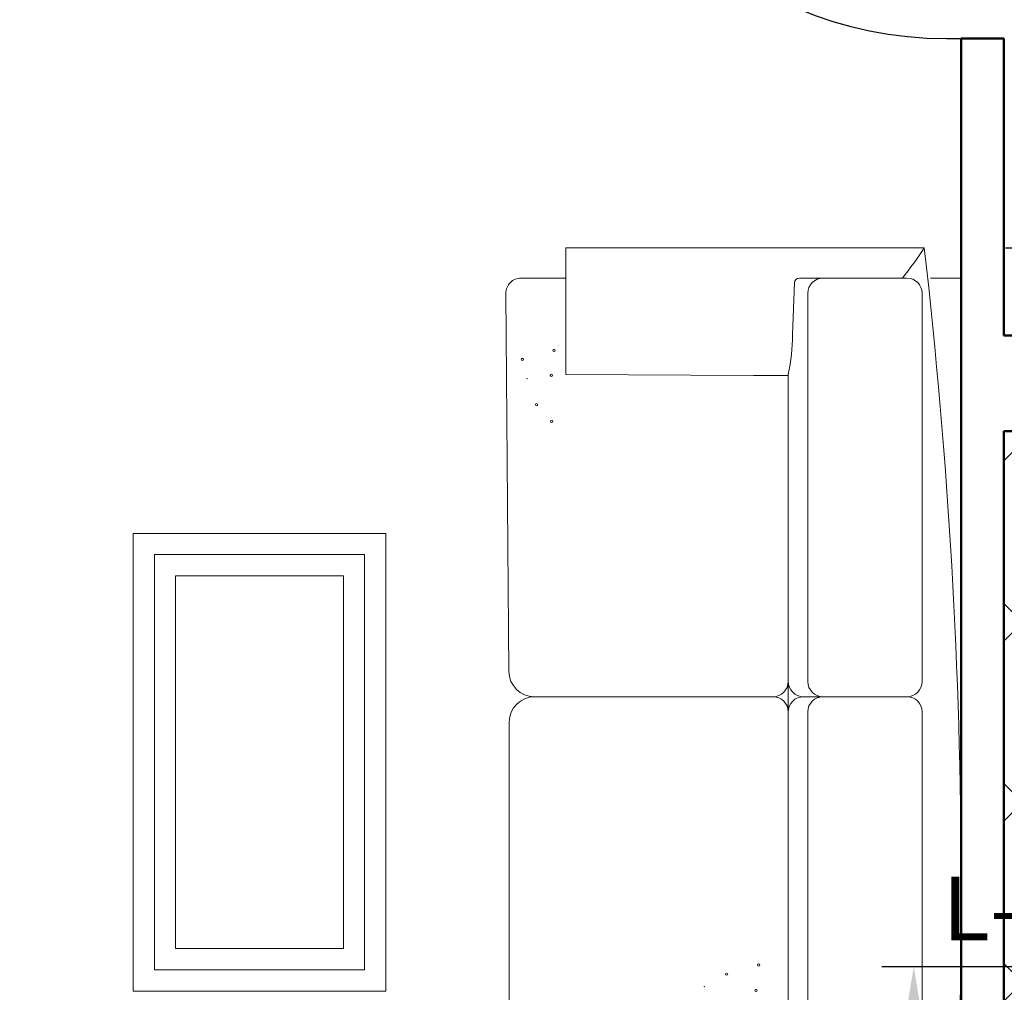
# Model space of a CAD drawing. Units: inches. Extents: x -466983 to 1020, y 324 to 318697.
# Tile 22 of 97: x 721 to 814, y 566 to 658. Entities that reach past the tile are written whole.
import ezdxf

# ---------------------------------------------------------------- set-up
doc = ezdxf.new("R2010")
doc.units = ezdxf.units.IN
doc.header["$MEASUREMENT"] = 0
for name, color, linetype, lineweight in [('A-ANNO-DIMS', 2, 'Continuous', 18), ('A-DOOR', 3, 'Continuous', 25), ('A-FLOR-PATT', 252, 'Continuous', 13), ('A-FURN', 8, 'Continuous', 18), ('A-WALL', 7, 'Continuous', 50)]:
    doc.layers.add(name, color=color, linetype=linetype, lineweight=lineweight)
doc.styles.get("Standard").update_dxf_attribs({"font": 'arial.ttf'})
doc.dimstyles.get("Standard").update_dxf_attribs({"dimtxt": 6, "dimasz": 4, "dimexe": 3, "dimexo": 3, "dimgap": 0.09, "dimtad": 0, "dimtih": 1, "dimtoh": 1, "dimdec": 1, "dimzin": 0, "dimdsep": 46, "dimlunit": 3, "dimtxsty": 'Standard', "dimcen": 0.09, "dimadec": 0, "dimazin": 0, "dimtfac": 1, "dimtdec": 1, "dimtofl": 0, "dimtmove": 0, "dimatfit": 3, "dimfxl": 1, "dimtolj": 1, "dimtzin": 0, "dimarcsym": 0})

# ---------------------------------------------------------------- blocks, each defined once
blk = doc.blocks.new('L Shaped Sofa')
at = {"ltscale": 2}
for p, q in [((2438.01, 846.521), (2438.01, 834.581)), ((2471.772, 846.521), (2438.01, 846.521)), ((2438.01, 843.655), (2433.801, 843.655)), ((2459.543, 843.195), (2459.371, 838.325)), ((2460.02, 843.655), (2462.233, 843.655)), ((2470.142, 843.655), (2462.233, 843.655)), ((2475.263, 843.655), (2472.363, 843.655)), ((2475.263, 843.655), (2475.263, 821.686)), ((2432.653, 806.575), (2432.368, 842.211)), ((2460.8, 842.223), (2460.8, 821.686)), ((2471.575, 842.223), (2471.575, 821.686)), ((2455.692, 834.489), (2438.01, 834.581)), ((2455.692, 834.489), (2458.96, 834.489)), ((2458.96, 834.581), (2458.96, 805.639)), ((2460.8, 805.639), (2460.8, 821.686)), ((2471.575, 805.639), (2471.575, 821.686)), ((2475.263, 723.229), (2475.263, 821.686)), ((2458.96, 802.773), (2458.96, 805.639)), ((2435.071, 804.206), (2435.04, 804.206)), ((2457.527, 804.206), (2435.071, 804.206)), ((2457.527, 804.206), (2457.527, 804.206)), ((2462.233, 804.206), (2460.393, 804.206)), ((2470.142, 804.206), (2462.233, 804.206)), ((2458.96, 739.532), (2458.96, 802.773)), ((2460.8, 737.692), (2460.8, 802.773)), ((2471.575, 769.955), (2471.575, 802.773)), ((2432.683, 769.955), (2432.683, 801.818))]:
    blk.add_line(p, q, dxfattribs=at)
for centre, radius, start, end in [((2441.545, 866.112), 36.021, 321.43275, 327.0519), ((1939.075, 785.436), 536.188, 353.68225, 6.54157), ((2433.801, 842.223), 1.433, 90, 180.45787), ((2460.02, 843.178), 0.478, 90, 177.98163), ((2462.233, 842.223), 1.433, 90, 180), ((2470.142, 842.223), 1.433, 0, 90), ((2441.716, 838.368), 17.655, 347.61307, 359.85818), ((2436.906, 836.857), 0.106, 1.3946, 181.3946), ((2436.906, 836.857), 0.106, 181.3946, 1.3946), ((2433.902, 836.001), 0.106, 1.3946, 181.3946), ((2433.902, 836.001), 0.106, 181.3946, 1.3946), ((2434.341, 834.182), 0.0177, 1.3946, 181.3946), ((2434.341, 834.182), 0.0177, 181.3946, 1.3946), ((2436.655, 834.485), 0.106, 1.3946, 181.3946), ((2436.655, 834.485), 0.106, 181.3946, 1.3946), ((2435.251, 831.737), 0.106, 1.3946, 181.3946), ((2435.251, 831.737), 0.106, 181.3946, 1.3946), ((2436.686, 830.165), 0.106, 1.3946, 181.3946), ((2436.686, 830.165), 0.106, 181.3946, 1.3946), ((2435.04, 806.594), 2.388, 180.45787, 270), ((2457.527, 805.639), 1.433, 270, 0), ((2460.393, 805.639), 1.433, 180, 270), ((2462.233, 805.639), 1.433, 180, 270), ((2470.142, 805.639), 1.433, 270, 0), ((2435.071, 801.818), 2.388, 90, 180), ((2457.527, 802.773), 1.433, 0, 90), ((2460.393, 802.773), 1.433, 90, 180), ((2462.233, 802.773), 1.433, 90, 180), ((2470.142, 802.773), 1.433, 0, 90), ((2453.169, 778.058), 0.106, 1.3946, 181.3946), ((2456.173, 778.913), 0.106, 1.3946, 181.3946), ((2456.173, 778.913), 0.106, 181.3946, 1.3946), ((2453.169, 778.058), 0.106, 181.3946, 1.3946), ((2451.048, 776.875), 0.0177, 1.3946, 181.3946), ((2451.048, 776.875), 0.0177, 181.3946, 1.3946), ((2455.922, 776.541), 0.106, 1.3946, 181.3946), ((2455.922, 776.541), 0.106, 181.3946, 1.3946)]:
    blk.add_arc(centre, radius, start, end, dxfattribs=at)
blk = doc.blocks.new('*U39')
for p, q in [((0, 0), (0, -6)), ((-40, 0), (-40, -6))]:
    blk.add_line(p, q)
blk.add_lwpolyline([(0, 0), (0, 40), (-1.75, 40), (-1.75, 0)], close=True)
blk.add_arc((0, 0), 40, 90, 180)
blk = doc.blocks.new('*D69')
at = {"layer": 'A-ANNO-DIMS', "color": 0, "lineweight": -2, "transparency": 16777216}
for p, q in [((813.968, 636.229), (832.65, 636.229)), ((829.65, 632.229), (829.65, 577.152)), ((829.65, 515.686), (829.65, 570.763)), ((813.968, 511.686), (832.65, 511.686))]:
    blk.add_line(p, q, dxfattribs=at)
at = {"layer": 'A-ANNO-DIMS', "color": 0, "transparency": 16777216}
for points in [[(828.983, 632.229), (830.316, 632.229), (829.65, 636.229)], [(828.983, 515.686), (830.316, 515.686), (829.65, 511.686)]]:
    blk.add_solid(points, dxfattribs=at)
at = {"layer": 'Defpoints', "color": 0, "transparency": 16777216}
for p in [(810.968, 636.229), (829.65, 636.229), (810.968, 511.686)]:
    blk.add_point(p, dxfattribs=at)
at = {"layer": 'A-ANNO-DIMS', "color": 0, "transparency": 16777216, "insert": (829.65, 573.958), "char_height": 6, "attachment_point": 5}
blk.add_mtext('\\A1;L-SOFA 125', dxfattribs=at)
blk = doc.blocks.new('*D97')
at = {"layer": 'A-ANNO-DIMS', "color": 0, "lineweight": -2, "transparency": 16777216}
for p, q in [((823.929, 568.441), (802.329, 568.441)), ((805.329, 564.441), (805.329, 499.545)), ((805.329, 428.441), (805.329, 493.337)), ((823.929, 424.441), (802.329, 424.441))]:
    blk.add_line(p, q, dxfattribs=at)
at = {"layer": 'A-ANNO-DIMS', "color": 0, "transparency": 16777216}
for points in [[(804.662, 564.441), (805.996, 564.441), (805.329, 568.441)], [(804.662, 428.441), (805.996, 428.441), (805.329, 424.441)]]:
    blk.add_solid(points, dxfattribs=at)
at = {"layer": 'Defpoints', "color": 0, "transparency": 16777216}
for p in [(826.929, 568.441), (805.329, 424.441), (826.929, 424.441)]:
    blk.add_point(p, dxfattribs=at)
at = {"layer": 'A-ANNO-DIMS', "color": 0, "transparency": 16777216, "insert": (805.329, 496.441), "char_height": 6, "attachment_point": 5}
blk.add_mtext('\\A1;BIKE 144', dxfattribs=at)

msp = doc.modelspace()

# ---------------------------------------------------------------- hatches: boundary and pattern name
at = {"layer": 'A-FLOR-PATT', "transparency": 33554572}
h = msp.add_hatch(dxfattribs=at)
h.set_pattern_fill('ANSI37', color=256, scale=30)
h.set_pattern_definition([(45, (-1212.4137, -290.035), (-2.6516504, 2.6516504), []), (135, (-1212.4137, -290.035), (-2.6516504, -2.6516504), [])])
h.paths.add_polyline_path([(901.806, 1075.938), (900.614, 1075.938), (900.614, 1065.386), (899.391, 1065.386), (898.091, 1065.386), (892.836, 1058.71, -0.258377), (892.188, 1058.351), (879.985, 1058.351, -0.20177), (879.438, 1058.581), (874.081, 1065.386), (872.781, 1065.386), (871.558, 1065.386), (871.558, 1075.938), (813.806, 1075.938), (813.806, 1044.792), (832.395, 1044.792, -0.394795), (848.66, 1028.536), (848.66, 1009.938), (901.806, 1009.938), (901.806, 1015.938), (901.306, 1015.938), (871.306, 1015.938), (871.306, 1017.25), (871.334, 1017.25, -0.401453), (901.306, 1045.938), (901.806, 1045.938)])
edge = h.paths.add_edge_path(flags=16)
edge.add_line((847.773, 1068.949), (847.773, 1073.709))
edge.add_arc((849.227, 1073.709), 1.454, 90, 180, ccw=False)
edge.add_line((849.227, 1075.163), (864.492, 1075.163))
edge.add_arc((864.492, 1073.709), 1.454, 0, 90, ccw=False)
edge.add_line((865.946, 1073.709), (865.946, 1069.004))
edge.add_arc((832.645, 1068.976), 33.301, -20.61234, 0.04725, ccw=False)
edge.add_ellipse((856.859, 1058.48), major_axis=(0, 10.213), ratio=0.685919, start_angle=100.00884, end_angle=259.99116, ccw=False)
edge.add_arc((881.074, 1068.976), 33.301, 180.04725, 200.61234, ccw=False)
h.paths.add_polyline_path([(853.146, 1066.482), (853.146, 1066.453), (853.146, 1066.453, 0.433107), (852.917, 1066.685), (852.917, 1066.453), (853.146, 1066.453), (853.146, 1066.482), (853.088, 1066.612, 0.697939), (852.7, 1066.453), (852.7, 1066.453), (852.7, 1066.482), (852.917, 1067.001), (852.917, 1066.685, -0.396254)], flags=0)
h.paths.add_polyline_path([(861.019, 1066.482), (861.019, 1066.453), (861.019, 1066.453, 0.416404), (860.802, 1066.685), (860.802, 1066.453), (861.019, 1066.453), (861.019, 1066.482), (860.967, 1066.605, 0.713344), (860.573, 1066.453), (860.573, 1066.453), (860.573, 1066.482), (860.802, 1067.001), (860.802, 1066.685, -0.379973)], flags=0)
edge = h.paths.add_edge_path(flags=0)
edge.add_spline(control_points=[(861.13, 1065.785), (861.466, 1065.248), (861.613, 1065.016), (861.983, 1064.374), (862.192, 1063.944), (862.561, 1063.039), (862.721, 1062.563), (862.987, 1061.578), (863.092, 1061.069), (863.245, 1060.031), (863.293, 1059.503), (863.329, 1058.441), (863.318, 1057.908), (863.237, 1056.852), (863.166, 1056.329), (862.97, 1055.308), (862.843, 1054.81), (862.537, 1053.852), (862.357, 1053.393), (861.951, 1052.525), (861.725, 1052.117), (861.233, 1051.362), (860.967, 1051.016), (860.405, 1050.395), (860.108, 1050.12), (859.494, 1049.646), (859.176, 1049.448), (858.528, 1049.13), (858.197, 1049.011), (857.531, 1048.852), (857.196, 1048.812), (856.525, 1048.812), (856.189, 1048.852), (855.524, 1049.01), (855.193, 1049.129), (854.545, 1049.447), (854.227, 1049.645), (853.612, 1050.118), (853.316, 1050.393), (852.753, 1051.014), (852.487, 1051.36), (851.995, 1052.114), (851.769, 1052.523), (851.363, 1053.39), (851.183, 1053.85), (850.877, 1054.807), (850.75, 1055.305), (850.553, 1056.326), (850.483, 1056.849), (850.401, 1057.905), (850.39, 1058.438), (850.426, 1059.5), (850.473, 1060.028), (850.626, 1061.066), (850.732, 1061.575), (850.997, 1062.561), (851.157, 1063.036), (851.525, 1063.942), (851.734, 1064.371), (852.106, 1065.016), (852.254, 1065.25), (852.608, 1065.733)], knot_values=[3.915332, 3.915332, 3.915332, 3.915332, 4.013468, 4.013468, 4.175532, 4.175532, 4.337596, 4.337596, 4.49966, 4.49966, 4.661724, 4.661724, 4.823788, 4.823788, 4.985852, 4.985852, 5.147916, 5.147916, 5.30998, 5.30998, 5.472044, 5.472044, 5.634109, 5.634109, 5.796173, 5.796173, 5.958237, 5.958237, 6.120301, 6.120301, 6.282365, 6.282365, 6.444429, 6.444429, 6.606493, 6.606493, 6.768557, 6.768557, 6.930621, 6.930621, 7.092685, 7.092685, 7.254749, 7.254749, 7.416813, 7.416813, 7.578878, 7.578878, 7.740942, 7.740942, 7.903006, 7.903006, 8.06507, 8.06507, 8.227134, 8.227134, 8.389198, 8.389198, 8.551262, 8.551262, 8.65037, 8.65037, 8.65037, 8.65037], degree=3, periodic=0)
edge.add_line((852.642, 1065.785), (861.13, 1065.785))
edge = h.paths.add_edge_path(flags=0)
edge.add_ellipse((856.85, 1057.743), major_axis=(0, 7.792), ratio=0.687861, start_angle=0, end_angle=360)
h.paths.add_polyline_path([(848.863, 1069.389), (848.863, 1073.96, -0.414214), (849.954, 1075.051), (863.765, 1075.051, -0.414214), (864.856, 1073.96), (864.856, 1069.389, -0.388936), (864.524, 1069.027, -0.043561), (849.195, 1069.027, -0.388936)], flags=0)
h.paths.add_polyline_path([(853.101, 1068.112, -1), (852.677, 1068.112, -1)], flags=0)
edge = h.paths.add_edge_path(flags=0)
edge.add_ellipse((856.859, 1057.338), major_axis=(0, 2.207), ratio=0.657164, start_angle=0, end_angle=360)
h.paths.add_polyline_path([(861.041, 1068.112, -1), (860.618, 1068.112, -1)], flags=0)
edge = h.paths.add_edge_path()
edge.add_line((573.954, 1057.341), (573.954, 1075.938))
edge.add_line((573.954, 1075.938), (558.731, 1075.938))
edge.add_line((558.731, 1075.938), (558.731, 1065.386))
edge.add_line((558.731, 1065.386), (557.507, 1065.386))
edge.add_line((557.507, 1065.386), (556.207, 1065.386))
edge.add_line((556.207, 1065.386), (550.952, 1058.71))
edge.add_arc((550.304, 1059.116), 0.765, 270, 327.94832, ccw=False)
edge.add_line((550.304, 1058.351), (538.101, 1058.351))
edge.add_arc((538.101, 1059.116), 0.765, 224.3704, 270, ccw=False)
edge.add_line((537.555, 1058.581), (532.198, 1065.386))
edge.add_line((532.198, 1065.386), (530.898, 1065.386))
edge.add_line((530.898, 1065.386), (529.674, 1065.386))
edge.add_line((529.674, 1065.386), (529.674, 1075.938))
edge.add_line((529.674, 1075.938), (520.806, 1075.938))
edge.add_line((520.806, 1075.938), (520.806, 1045.938))
edge.add_line((520.806, 1045.938), (521.306, 1045.938))
edge.add_arc((521.306, 1015.938), 30, 2.50749, 90, ccw=False)
edge.add_line((551.277, 1017.25), (551.306, 1017.25))
edge.add_line((551.306, 1017.25), (551.306, 1015.938))
edge.add_line((551.306, 1015.938), (520.806, 1015.938))
edge.add_line((520.806, 1015.938), (520.806, 1009.938))
edge.add_line((520.806, 1009.938), (559.191, 1010.402))
edge.add_arc((559.191, 1011.856), 1.454, 180, 270, ccw=False)
edge.add_line((557.737, 1011.856), (557.737, 1016.561))
edge.add_arc((591.039, 1016.589), 33.301, 159.38766, 180.04725, ccw=False)
edge.add_ellipse((566.824, 1027.085), major_axis=(0, 10.213), ratio=0.685919, start_angle=280.00884, end_angle=439.99116, ccw=False)
edge.add_arc((542.609, 1016.589), 33.301, 0.04725, 20.61234, ccw=False)
edge.add_line((575.91, 1016.616), (575.91, 1011.856))
edge.add_arc((574.456, 1011.856), 1.454, -90, 0, ccw=False)
edge.add_line((574.456, 1010.402), (608.806, 1009.938))
edge.add_line((608.806, 1009.938), (608.806, 1041.086))
edge.add_line((608.806, 1041.086), (590.218, 1041.086))
edge.add_arc((590.775, 1057.907), 16.831, 181.92775, 268.10321, ccw=False)
edge = h.paths.add_edge_path()
edge.add_ellipse((494.244, 583.62), major_axis=(0, 10.213), ratio=0.685919, start_angle=280.00884, end_angle=439.99116, ccw=False)
edge.add_arc((470.03, 573.124), 33.301, 0.04725, 20.61234, ccw=False)
edge.add_line((503.331, 573.152), (503.331, 568.392))
edge.add_arc((501.877, 568.392), 1.454, -90, 0, ccw=False)
edge.add_line((501.877, 566.938), (539.806, 566.938))
edge.add_line((539.806, 566.938), (539.806, 572.938))
edge.add_line((539.806, 572.938), (539.306, 572.938))
edge.add_line((539.306, 572.938), (509.306, 572.938))
edge.add_line((509.306, 572.938), (509.306, 574.25))
edge.add_line((509.306, 574.25), (509.334, 574.25))
edge.add_arc((539.306, 572.938), 30, 90, 177.49251, ccw=False)
edge.add_line((539.306, 602.938), (539.806, 602.938))
edge.add_line((539.806, 602.938), (539.806, 626.938))
edge.add_line((539.806, 626.938), (531.772, 626.938))
edge.add_line((531.772, 626.938), (531.772, 616.386))
edge.add_line((531.772, 616.386), (530.548, 616.386))
edge.add_line((530.548, 616.386), (529.249, 616.386))
edge.add_line((529.249, 616.386), (523.711, 609.351))
edge.add_line((523.711, 609.351), (510.777, 609.351))
edge.add_line((510.777, 609.351), (505.239, 616.386))
edge.add_line((505.239, 616.386), (503.939, 616.386))
edge.add_line((503.939, 616.386), (502.715, 616.386))
edge.add_line((502.715, 616.386), (502.715, 626.938))
edge.add_line((502.715, 626.938), (481.698, 626.938))
edge.add_line((481.698, 626.938), (481.698, 610.995))
edge.add_arc((467.27, 611.473), 14.436, 271.92775, 358.10321, ccw=False)
edge.add_line((467.756, 597.045), (451.806, 597.045))
edge.add_line((451.806, 597.045), (451.806, 584.404))
edge.add_line((451.806, 584.404), (451.806, 566.938))
edge.add_line((451.806, 566.938), (486.612, 566.938))
edge.add_arc((486.612, 568.392), 1.454, 180, 270, ccw=False)
edge.add_line((485.158, 568.392), (485.158, 573.097))
edge.add_arc((518.459, 573.124), 33.301, 159.38766, 180.04725, ccw=False)
h.paths.add_polyline_path([(836.261, 1020.733), (879.89, 1020.733), (879.89, 1039.39), (836.261, 1039.39)], flags=25)
h.paths.add_polyline_path([(549.985, 1036.749), (593.614, 1036.749), (593.614, 1055.407), (549.985, 1055.407)], flags=24)
h.paths.add_polyline_path([(475.123, 595.596), (518.752, 595.596), (518.752, 614.253), (475.123, 614.253)], flags=24)
h = msp.add_hatch(dxfattribs=at)
h.set_pattern_fill('AR-HBONE', color=256, scale=3)
h.set_pattern_definition([(45, (-1212.414, -290.035), (0, 16.97056), [36, -12]), (135, (-1203.928, -281.55), (1e-15, 16.97056), [36, -12])])
h.paths.add_polyline_path([(987.806, 618.938), (813.806, 618.938), (813.806, 368.938), (987.806, 368.938)])

# ---------------------------------------------------------------- linework, layer by layer
at = {"layer": 'A-FURN'}
for points in [[(731.798, 609.305), (755.602, 609.305), (755.602, 566.168), (731.798, 566.168)], [(733.798, 607.305), (753.602, 607.305), (753.602, 568.168), (733.798, 568.168)], [(735.798, 605.305), (751.602, 605.305), (751.602, 570.168), (735.798, 570.168)]]:
    msp.add_lwpolyline(points, close=True, dxfattribs=at)
at = {"layer": 'A-WALL'}
for p, q in [((813.806, 655.938), (809.806, 655.938)), ((809.806, 655.938), (809.806, 512.938)), ((813.806, 655.938), (813.806, 627.938)), ((934.806, 627.938), (813.806, 627.938)), ((813.806, 618.938), (813.806, 368.938)), ((934.806, 618.938), (813.806, 618.938))]:
    msp.add_line(p, q, dxfattribs=at)

# ---------------------------------------------------------------- block references
at = {"layer": 'A-DOOR', "xscale": 0.9000000000000035, "yscale": 0.9000000000000035, "zscale": 0.9000000000000035, "rotation": 90}
msp.add_blockref('*U39', (808.406, 691.938), dxfattribs=at)
at = {"layer": 'A-FURN'}
msp.add_blockref('L Shaped Sofa', (-1665.457, -210.292), dxfattribs=at)

# ---------------------------------------------------------------- dimensions: what is measured, and where the dimension line sits
at = {"layer": 'A-ANNO-DIMS'}
for base, p1, p2, angle, text, picture, middle in [((829.65, 636.229), (810.968, 511.686), (810.968, 636.229), 90, 'L-SOFA <>', '*D69', (829.65, 573.958)), ((805.329, 424.441), (826.929, 568.441), (826.929, 424.441), 270, 'BIKE <>', '*D97', (805.329, 496.441))]:
    dim = msp.add_linear_dim(base=base, p1=p1, p2=p2, angle=angle, text=text, dimstyle='Standard', override={"dimdec": 0, "dimlfac": 1, "dimrnd": 0, "dimzin": 0, "dimdsep": 46, "dimlunit": 2}, dxfattribs=at)
    dim.commit()
    dim.dimension.update_dxf_attribs({"geometry": picture, "text_midpoint": middle})

doc.saveas('drawing.dxf')
